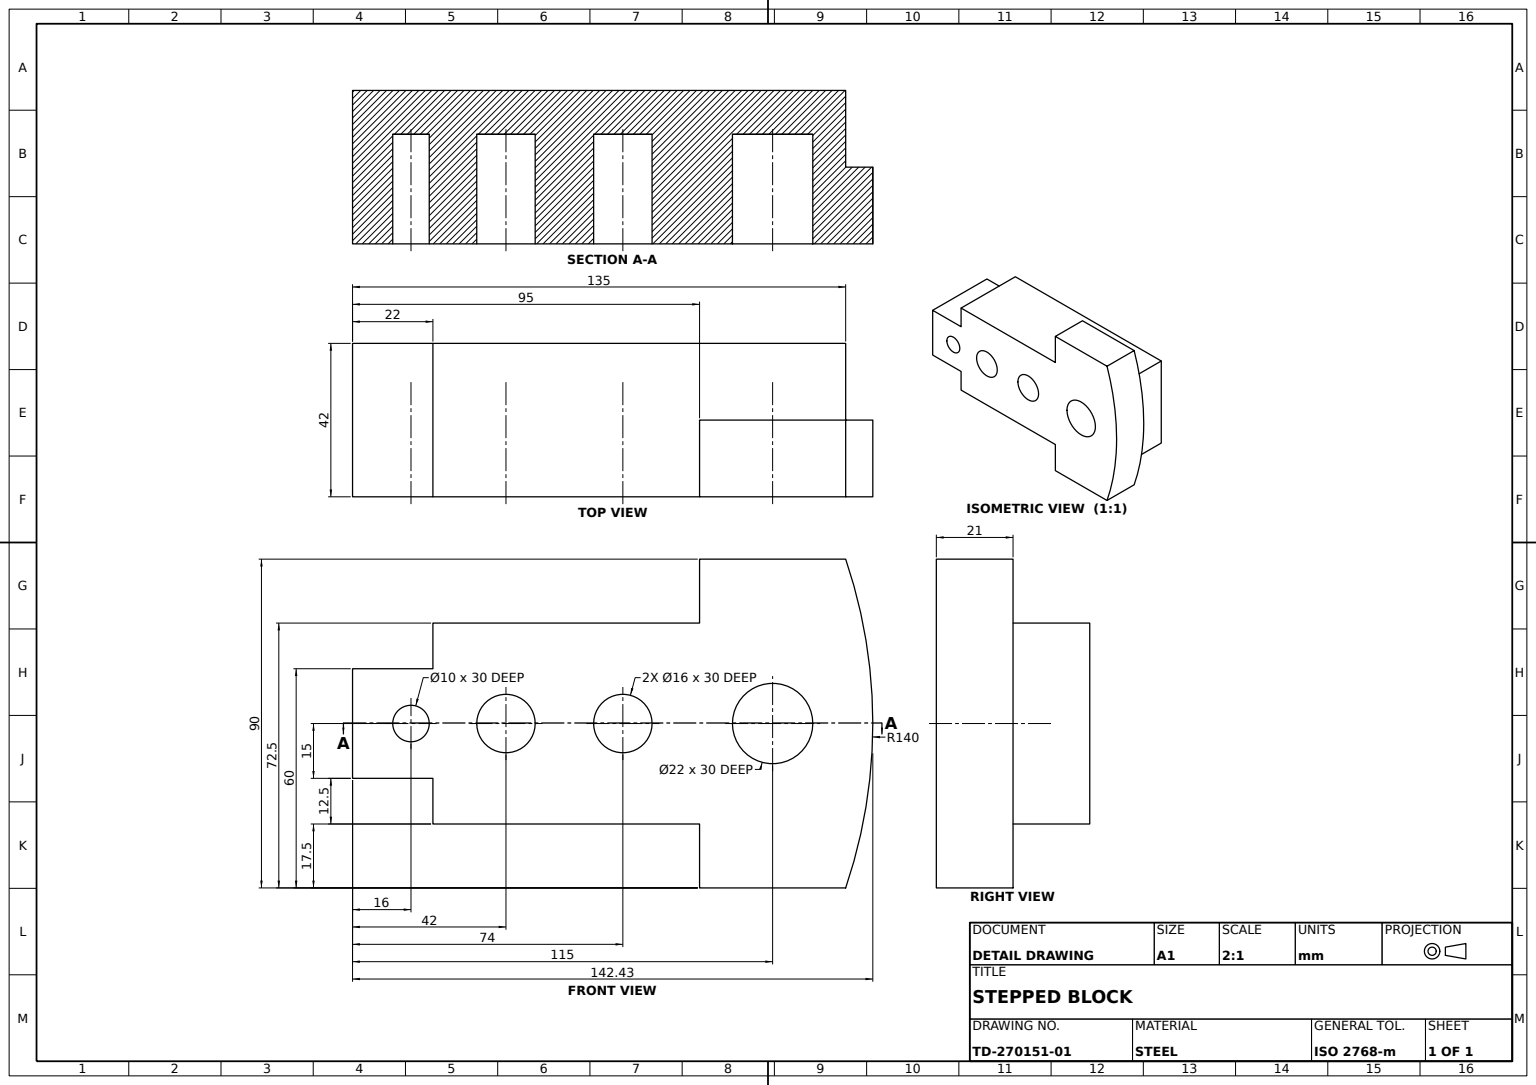
SolidWorks part; units mm, degrees
material "Plain Carbon Steel"
ref_plane "Front Plane" through (0, 0, 0) normal (0, 0, 1) x (1, 0, 0)
ref_plane "Top Plane" through (0, 0, 0) normal (0, 1, 0) x (1, 0, 0)
ref_plane "Right Plane" through (0, 0, 0) normal (1, 0, 0) x (0, 0, -1)
sketch "Base Profile Sketch" plane through (0, 0, 0) normal (0, 0, 1) x (1, 0, 0)
  line L0 (0, 0) -> (115, 0)
  line L1 (115, 0) -> (115, 90)
  line L2 (115, 90) -> (54, 90)
  line L3 (54, 90) -> (22, 90)
  line L4 (22, 90) -> (-4, 90)
  line L5 (-4, 90) -> (-4, 0)
  line L6 (-4, 0) -> (0, 0)
  dimension "D1" = 4
  dimension "D2" = 26
  dimension "D3" = 58
  dimension "D4" = 119
  dimension "D5" = 90
extrude "Base Block 63mm" add sketch "Base Profile Sketch" along normal blind 63
sketch "Profile Cut Sketch" plane through (0, 0, 63) normal (0, 0, 1) x (1, 0, 0)
  line L0 (18, 72.5) -> (18, 90)
  line L1 (-4, 90) -> (-4, 0) construction
  line L6 (18, 17.5) -> (18, 0)
  line L7 (-4, 0) -> (115, 0) construction
  line L8 (18, 0) -> (18, 17.5)
  line L9 (115, 90) -> (-4, 90) construction
  line L10 (18, 90) -> (-4, 90)
  line L11 (-4, 90) -> (-4, 72.5)
  line L12 (-4, 17.5) -> (-4, 0)
  line L13 (-4, 0) -> (18, 0)
  line L15 (-4, 60) -> (18, 60)
  line L17 (18, 30) -> (-4, 30)
  line L19 (18, 72.5) -> (18, 60)
  line L20 (-4, 72.5) -> (-4, 60)
  line L21 (18, 17.5) -> (18, 30)
  line L22 (-4, 17.5) -> (-4, 30)
  line L23 (115, 0) -> (115, 90) construction
  line M1 (-4, 0) -> (115, 0)
  line M3 (115, 90) -> (-4, 90)
  line M4 (-4, 90) -> (-4, 0)
  dimension "D1" = 97
  dimension "D2" = 17.5
  dimension "D3" = 30
extrude "Profile Cut 63mm" cut sketch "Profile Cut Sketch" against normal blind 63 contours L19 L0 L15 M3 M4 | L6 L21 L17 M4 M1
sketch "Side Boss Sketch" plane through (115, 0, 0) normal (1, 0, 0) x (0, 0, -1)
  line L0 (-63, 90) -> (0, 90)
  line L1 (0, 90) -> (0, 0)
  line L2 (0, 0) -> (-63, 0)
  line L3 (-63, 0) -> (-63, 90)
extrude "Side Boss 16mm" add sketch "Side Boss Sketch" along normal blind 16
sketch "Step Cut Sketch" plane through (0, 0, 63) normal (0, 0, 1) x (1, 0, 0)
  line L0 (18, 90) -> (91, 90)
  line L2 (91, 0) -> (18, 0)
  line L3 (18, 30) -> (18, 0) construction
  line L4 (18, 0) -> (18, 30)
  line L5 (18, 30) -> (-4, 30)
  line L6 (-4, 30) -> (-4, 60)
  line L7 (-4, 60) -> (18, 60) construction
  line L8 (-4, 60) -> (-4, 30) construction
  line L9 (-4, 60) -> (18, 60)
  line L10 (18, 60) -> (18, 90)
  line L11 (91, 90) -> (131, 90)
  line L14 (131, 90) -> (131, 0)
  line L15 (131, 0) -> (91, 0)
  dimension "D1" = 95
extrude "Step Cut 21mm" cut sketch "Step Cut Sketch" against normal blind 21
sketch "Curved End Boss Sketch" plane through (0, 0, 42) normal (0, 0, 1) x (1, 0, 0)
  line L0 (131, 90) -> (131, 0)
  arc A0 (131, 90) -> (131, 0) centre (-1.5707, 45) cw
  dimension "D1" = 140
extrude "Curved End Boss 21mm" add sketch "Curved End Boss Sketch" against normal blind 21
sketch "Pocket Cut Sketch" plane through (131, 0, 0) normal (1, 0, 0) x (0, 0, -1)
  line L1 (0, 0) -> (0, 90) construction
  line L2 (0, 72.5) -> (-21, 72.5)
  line L3 (-21, 90) -> (-21, 0) construction
  line L5 (-21, 17.5) -> (0, 17.5)
  line L7 (-21, 90) -> (0, 90)
  line L8 (0, 90) -> (0, 72.5)
  line L9 (0, 72.5) -> (-21, 72.5)
  line L10 (-21, 17.5) -> (-21, 0)
  line L11 (-21, 0) -> (0, 0)
  line L12 (0, 0) -> (0, 17.5)
  line L13 (-21, 90) -> (-21, 72.5)
  line L14 (0, 90) -> (-21, 90) construction
  line M1 (0, 90) -> (-21, 90)
  line M2 (-21, 90) -> (-21, 0)
  line M3 (-21, 0) -> (0, 0)
  line M4 (0, 0) -> (0, 90)
  dimension "D1" = 17.5
extrude "Pocket Cut 40mm" cut sketch "Pocket Cut Sketch" against normal blind 40 contours L2 M4 M1 M2 | L5 M2 M3 M4
sketch "Hole A Sketch" plane through (0, 0, 0) normal (0, -1, 0) x (1, 0, 0)
  line L0 (18, 42) -> (91, 42)
  line L1 (18, 42) -> (131, 42) construction
  line L2 (91, 42) -> (91, 0)
  line L3 (91, 0) -> (18, 0)
  line L4 (18, 0) -> (18, 42)
extrude "Hole A 17.5mm Deep" cut sketch "Hole A Sketch" against normal blind 17.5
sketch "Hole B Sketch" plane through (0, 90, 0) normal (0, 1, 0) x (1, 0, 0)
  line L0 (18, 0) -> (91, 0)
  line L1 (91, 0) -> (91, -42)
  line L2 (131, -42) -> (18, -42) construction
  line L3 (91, -42) -> (18, -42)
  line L4 (18, -42) -> (18, 0)
extrude "Hole B 17.5mm Deep" cut sketch "Hole B Sketch" against normal blind 17.5
sketch "End Cut Sketch" plane through (0, 0, 42) normal (0, 0, 1) x (1, 0, 0)
  line L0 (-4, 60) -> (-4, 30) construction
  line L1 (131, 90) -> (91, 90) construction
  circle A0 centre (111, 45) radius 11
  circle A1 centre (70, 45) radius 8
  circle A2 centre (38, 45) radius 8
  circle A3 centre (12, 45) radius 5
  dimension "D1" = 10
  dimension "D2" = 16
  dimension "D3" = 22
  dimension "D4" = 16
  dimension "D5" = 42
  dimension "D6" = 74
  dimension "D7" = 115
  dimension "D8" = 45
extrude "End Cut 30mm" cut sketch "End Cut Sketch" against normal blind 30
